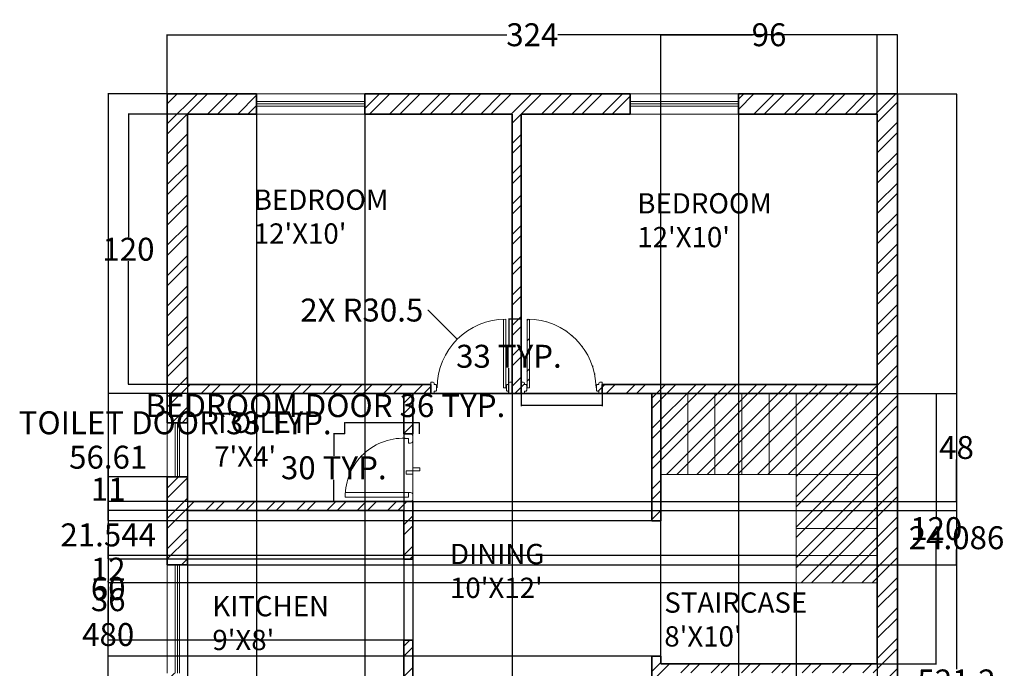
# Model space of a CAD drawing. Units: inches. Extents: x 2025 to 2472, y 2991 to 3578.
# Tile 2 of 2: x 2025 to 2462, y 3291 to 3578. Entities that reach past the tile are written whole.
import ezdxf

# ---------------------------------------------------------------- set-up
doc = ezdxf.new("R2010")
doc.units = ezdxf.units.IN
for name, color, linetype, lineweight in [('00 FURNITURE', 15, 'Continuous', 15), ('A-ANNO-DIMS', 2, 'Continuous', 18), ('A-AREA-IDEN', 7, 'Continuous', 18), ('A-DOOR', 4, 'Continuous', 18), ('A-FLOR-STRS', 7, 'Continuous', 18), ('A-WALL-PATT', 252, 'Continuous', 13), ('A_FUR 1', 5, 'Continuous', 5), ('WALL', 7, 'Continuous', 35), ('WINDOW', 160, 'Continuous', 13)]:
    doc.layers.add(name, color=color, linetype=linetype, lineweight=lineweight)
doc.styles.get("Standard").update_dxf_attribs({"font": 'arial.ttf'})
doc.dimstyles.get("Standard").update_dxf_attribs({"dimtxt": 10.18, "dimasz": 0.18, "dimexe": 0.18, "dimexo": 0.0625, "dimgap": 0.09, "dimtad": 0, "dimtih": 1, "dimtoh": 1, "dimdec": 0, "dimzin": 0, "dimdsep": 46, "dimlunit": 3, "dimtxsty": 'Standard', "dimcen": 0.09, "dimadec": 0, "dimazin": 0, "dimtfac": 1, "dimtdec": 0, "dimtofl": 0, "dimtmove": 0, "dimatfit": 3, "dimfxl": 1, "dimtolj": 1, "dimtzin": 0, "dimarcsym": 0})

# ---------------------------------------------------------------- blocks, each defined once
blk = doc.blocks.new('DDD')
at = {"layer": '00 FURNITURE'}
for p, q in [((-12579.77, -15859.53), (-12579.77, -15829.05)), ((-12578.77, -15859.53), (-12578.77, -15829.03)), ((-12612.02, -15857.03), (-12612.02, -15862.03)), ((-12611.02, -15857.03), (-12612.02, -15857.03)), ((-12610.52, -15858.03), (-12610.52, -15857.53)), ((-12577.52, -15858.03), (-12577.52, -15857.53)), ((-12577.02, -15857.03), (-12576.02, -15857.03)), ((-12576.02, -15857.03), (-12576.02, -15862.03)), ((-12612.02, -15862.03), (-12611.02, -15862.03)), ((-12610.52, -15861.53), (-12610.52, -15861.03)), ((-12578.77, -15859.53), (-12579.77, -15859.53)), ((-12577.52, -15861.53), (-12577.52, -15861.03)), ((-12576.02, -15862.03), (-12577.02, -15862.03))]:
    blk.add_line(p, q, dxfattribs=at)
for points in [[(-12610.52, -15861.03), (-12610.02, -15861.03, 0.414214), (-12609.52, -15860.53), (-12609.52, -15858.53, 0.414214), (-12610.02, -15858.03), (-12610.52, -15858.03)], [(-12577.52, -15861.03), (-12578.02, -15861.03, -0.414214), (-12578.52, -15860.53), (-12578.52, -15858.53, -0.414214), (-12578.02, -15858.03), (-12577.52, -15858.03)]]:
    blk.add_lwpolyline(points, format="xyb", dxfattribs=at)
for centre, radius, start, end in [((-12578.77, -15859.53), 30.5, 90, 180), ((-12611.02, -15857.53), 0.5, 0, 90), ((-12577.02, -15857.53), 0.5, 90, 180), ((-12611.02, -15861.53), 0.5, 270, 0), ((-12577.02, -15861.53), 0.5, 180, 270)]:
    blk.add_arc(centre, radius, start, end, dxfattribs=at)
blk = doc.blocks.new('ESTSET')
at = {"layer": 'A_FUR 1'}
for p, q in [((-10.44, 4.1), (-10.44, 32.1)), ((-8.44, 4.1), (-8.44, 32.1)), ((-36.44, 6.1), (-36.44, 3.1)), ((-34.44, 6.1), (-36.44, 6.1)), ((-34.44, 4.1), (-34.44, 6.1)), ((-34.44, 4.1), (-34.44, 6.1)), ((-8.44, 4.1), (-8.44, 6.1)), ((-8.44, 6.1), (-6.44, 6.1)), ((-8.44, 4.1), (-8.44, 6.1)), ((-6.44, 6.1), (-6.44, 3.1)), ((-6.44, 2.1), (-36.44, 2.1)), ((-35.44, 2.1), (-33.44, 2.1)), ((-32.44, 4.1), (-34.44, 4.1)), ((-32.44, 4.1), (-34.44, 4.1)), ((-32.44, 3.1), (-32.44, 4.1)), ((-10.44, 3.1), (-10.44, 4.1)), ((-10.44, 4.1), (-8.44, 4.1)), ((-10.44, 4.1), (-8.44, 4.1)), ((-7.44, 2.1), (-9.44, 2.1))]:
    blk.add_line(p, q, dxfattribs=at)
for points in [[(-21.44, 2.1), (-18.67, 2.1), (-18.67, 5.1), (-20.06, 5.1)], [(-20.06, 5.1), (-20.06, -0.91)], [(-21.44, 2.1), (-21.44, -0.91), (-20.06, -0.91)]]:
    blk.add_lwpolyline(points, dxfattribs=at)
for centre, radius, start, end in [((-8.91, 6.46), 25.64, 88.9606, 185.2816), ((-35.44, 3.1), 1, 180, 270), ((-33.44, 3.1), 1, 270, 0), ((-9.44, 3.1), 1, 180, 270), ((-7.44, 3.1), 1, 270, 0)]:
    blk.add_arc(centre, radius, start, end, dxfattribs=at)
blk = doc.blocks.new('WIN-48IN')
for p, q in [((48, 9), (0, 9)), ((48, 5.5), (0, 5.5)), ((48, 4.5), (0, 4.5)), ((48, 3.5), (0, 3.5)), ((0, 0), (48, 0))]:
    blk.add_line(p, q)
blk = doc.blocks.new('WIN-24IN')
for p, q in [((3.5, 24), (3.5, 0)), ((4.5, 24), (4.5, 0)), ((5.5, 24), (5.5, 0))]:
    blk.add_line(p, q)
blk.add_lwpolyline([(0, 0), (9, 0), (9, 24), (0, 24)], close=True)
blk = doc.blocks.new('*D10')
at = {"layer": 'A-ANNO-DIMS', "color": 0, "lineweight": -2, "transparency": 16777216}
for p, q in [((2247.79, 3412.44), (2247.79, 3406.92)), ((2283.79, 3412.44), (2283.79, 3406.92)), ((2247.79, 3407.1), (2247.61, 3407.1)), ((2283.61, 3407.1), (2247.97, 3407.1))]:
    blk.add_line(p, q, dxfattribs=at)
at = {"layer": 'A-ANNO-DIMS', "color": 0, "transparency": 16777216}
for points in [[(2247.97, 3407.13), (2247.97, 3407.07), (2247.79, 3407.1)], [(2283.61, 3407.13), (2283.61, 3407.07), (2283.79, 3407.1)]]:
    blk.add_solid(points, dxfattribs=at)
at = {"layer": 'Defpoints', "color": 0, "transparency": 16777216}
for p in [(2247.79, 3412.5), (2283.79, 3412.5), (2247.79, 3407.1)]:
    blk.add_point(p, dxfattribs=at)
at = {"layer": 'A-ANNO-DIMS', "color": 0, "transparency": 16777216, "insert": (2160.94, 3407.1), "char_height": 10.18, "attachment_point": 5}
blk.add_mtext('\\A1;BEDROOM DOOR 36 TYP.', dxfattribs=at)
blk = doc.blocks.new('*D11')
at = {"layer": 'A-ANNO-DIMS', "color": 0, "lineweight": -2, "transparency": 16777216}
for p, q in [((2247.72, 3445.5), (2242.21, 3445.5)), ((2242.39, 3445.32), (2242.39, 3434.29)), ((2242.39, 3412.68), (2242.39, 3423.71)), ((2247.72, 3412.5), (2242.21, 3412.5))]:
    blk.add_line(p, q, dxfattribs=at)
at = {"layer": 'A-ANNO-DIMS', "color": 0, "transparency": 16777216}
for points in [[(2242.36, 3445.32), (2242.42, 3445.32), (2242.39, 3445.5)], [(2242.36, 3412.68), (2242.42, 3412.68), (2242.39, 3412.5)]]:
    blk.add_solid(points, dxfattribs=at)
at = {"layer": 'Defpoints', "color": 0, "transparency": 16777216}
for p in [(2242.39, 3445.5), (2247.79, 3445.5), (2247.79, 3412.5)]:
    blk.add_point(p, dxfattribs=at)
at = {"layer": 'A-ANNO-DIMS', "color": 0, "transparency": 16777216, "insert": (2242.39, 3429), "char_height": 10.18, "attachment_point": 5}
blk.add_mtext('\\A1;33 TYP.', dxfattribs=at)
blk = doc.blocks.new('*D12')
at = {"layer": 'A-ANNO-DIMS', "color": 0, "lineweight": -2, "transparency": 16777216}
for p, q in [((2169.65, 3399.47), (2169.47, 3399.47)), ((2169.65, 3394.56), (2169.65, 3399.65)), ((2202.61, 3399.47), (2169.83, 3399.47)), ((2202.79, 3394.56), (2202.79, 3399.65))]:
    blk.add_line(p, q, dxfattribs=at)
at = {"layer": 'A-ANNO-DIMS', "color": 0, "transparency": 16777216}
for points in [[(2169.83, 3399.5), (2169.83, 3399.44), (2169.65, 3399.47)], [(2202.61, 3399.5), (2202.61, 3399.44), (2202.79, 3399.47)]]:
    blk.add_solid(points, dxfattribs=at)
at = {"layer": 'Defpoints', "color": 0, "transparency": 16777216}
for p in [(2169.65, 3399.47), (2169.65, 3394.5), (2202.79, 3394.5)]:
    blk.add_point(p, dxfattribs=at)
at = {"layer": 'A-ANNO-DIMS', "color": 0, "transparency": 16777216, "insert": (2094.3, 3399.47), "char_height": 10.18, "attachment_point": 5}
blk.add_mtext('\\A1;TOILET DOOR 33 TYP.', dxfattribs=at)
blk = doc.blocks.new('*D13')
at = {"layer": 'A-ANNO-DIMS', "color": 0, "lineweight": -2, "transparency": 16777216}
for p, q in [((2169.59, 3394.5), (2164.5, 3394.5)), ((2164.68, 3394.32), (2164.68, 3384.79)), ((2164.68, 3364.68), (2164.68, 3374.21)), ((2169.59, 3364.5), (2164.5, 3364.5))]:
    blk.add_line(p, q, dxfattribs=at)
at = {"layer": 'A-ANNO-DIMS', "color": 0, "transparency": 16777216}
for points in [[(2164.65, 3394.32), (2164.71, 3394.32), (2164.68, 3394.5)], [(2164.65, 3364.68), (2164.71, 3364.68), (2164.68, 3364.5)]]:
    blk.add_solid(points, dxfattribs=at)
at = {"layer": 'Defpoints', "color": 0, "transparency": 16777216}
for p in [(2169.65, 3394.5), (2164.68, 3364.5), (2169.65, 3364.5)]:
    blk.add_point(p, dxfattribs=at)
at = {"layer": 'A-ANNO-DIMS', "color": 0, "transparency": 16777216, "insert": (2164.68, 3379.5), "char_height": 10.18, "attachment_point": 5}
blk.add_mtext('\\A1;30 TYP.', dxfattribs=at)
blk = doc.blocks.new('*D14')
at = {"layer": 'A-ANNO-DIMS', "color": 0, "lineweight": -2, "transparency": 16777216}
for p, q in [((2090.79, 3545.56), (2090.79, 3571.88)), ((2090.97, 3571.7), (2241.47, 3571.7)), ((2414.61, 3571.7), (2264.1, 3571.7)), ((2414.79, 3545.56), (2414.79, 3571.88))]:
    blk.add_line(p, q, dxfattribs=at)
at = {"layer": 'A-ANNO-DIMS', "color": 0, "transparency": 16777216}
for points in [[(2090.97, 3571.73), (2090.97, 3571.67), (2090.79, 3571.7)], [(2414.61, 3571.73), (2414.61, 3571.67), (2414.79, 3571.7)]]:
    blk.add_solid(points, dxfattribs=at)
at = {"layer": 'Defpoints', "color": 0, "transparency": 16777216}
for p in [(2414.79, 3571.7), (2090.79, 3545.5), (2414.79, 3545.5)]:
    blk.add_point(p, dxfattribs=at)
at = {"layer": 'A-ANNO-DIMS', "color": 0, "transparency": 16777216, "insert": (2252.79, 3571.7), "char_height": 10.18, "attachment_point": 5}
blk.add_mtext('\\A1;324', dxfattribs=at)
blk = doc.blocks.new('*D15')
at = {"layer": 'A-ANNO-DIMS', "color": 0, "lineweight": -2, "transparency": 16777216}
for p, q in [((2414.85, 3545.5), (2441.17, 3545.5)), ((2440.99, 3545.32), (2440.99, 3290.19)), ((2440.99, 3024.48), (2440.99, 3279.61)), ((2267.85, 3024.3), (2441.17, 3024.3))]:
    blk.add_line(p, q, dxfattribs=at)
at = {"layer": 'A-ANNO-DIMS', "color": 0, "transparency": 16777216}
for points in [[(2440.96, 3545.32), (2441.02, 3545.32), (2440.99, 3545.5)], [(2440.96, 3024.48), (2441.02, 3024.48), (2440.99, 3024.3)]]:
    blk.add_solid(points, dxfattribs=at)
at = {"layer": 'Defpoints', "color": 0, "transparency": 16777216}
for p in [(2414.79, 3545.5), (2440.99, 3545.5), (2267.79, 3024.3)]:
    blk.add_point(p, dxfattribs=at)
at = {"layer": 'A-ANNO-DIMS', "color": 0, "transparency": 16777216, "insert": (2440.99, 3284.9), "char_height": 10.18, "attachment_point": 5}
blk.add_mtext('\\A1;521.2', dxfattribs=at)
blk = doc.blocks.new('*D16')
at = {"layer": 'A-ANNO-DIMS', "color": 0, "lineweight": -2, "transparency": 16777216}
for p, q in [((2090.72, 3545.5), (2064.41, 3545.5)), ((2064.59, 3545.32), (2064.59, 3310.79)), ((2064.59, 3065.68), (2064.59, 3300.21)), ((2090.72, 3065.5), (2064.41, 3065.5))]:
    blk.add_line(p, q, dxfattribs=at)
at = {"layer": 'A-ANNO-DIMS', "color": 0, "transparency": 16777216}
for points in [[(2064.56, 3545.32), (2064.62, 3545.32), (2064.59, 3545.5)], [(2064.56, 3065.68), (2064.62, 3065.68), (2064.59, 3065.5)]]:
    blk.add_solid(points, dxfattribs=at)
at = {"layer": 'Defpoints', "color": 0, "transparency": 16777216}
for p in [(2064.59, 3545.5), (2090.79, 3545.5), (2090.79, 3065.5)]:
    blk.add_point(p, dxfattribs=at)
at = {"layer": 'A-ANNO-DIMS', "color": 0, "transparency": 16777216, "insert": (2064.59, 3305.5), "char_height": 10.18, "attachment_point": 5}
blk.add_mtext('\\A1;480', dxfattribs=at)
blk = doc.blocks.new('*D18')
at = {"layer": 'A-ANNO-DIMS', "color": 0, "lineweight": -2, "transparency": 16777216}
for p, q in [((2099.79, 3536.44), (2099.79, 2997.92)), ((2130.46, 3536.44), (2130.46, 2997.92)), ((2099.97, 2998.1), (2130.28, 2998.1)), ((2130.46, 2998.1), (2130.64, 2998.1))]:
    blk.add_line(p, q, dxfattribs=at)
at = {"layer": 'A-ANNO-DIMS', "color": 0, "transparency": 16777216}
for points in [[(2099.97, 2998.13), (2099.97, 2998.07), (2099.79, 2998.1)], [(2130.28, 2998.13), (2130.28, 2998.07), (2130.46, 2998.1)]]:
    blk.add_solid(points, dxfattribs=at)
at = {"layer": 'Defpoints', "color": 0, "transparency": 16777216}
for p in [(2099.79, 3536.5), (2130.46, 3536.5), (2130.46, 2998.1)]:
    blk.add_point(p, dxfattribs=at)
at = {"layer": 'A-ANNO-DIMS', "color": 0, "transparency": 16777216, "insert": (2151.86, 2998.1), "char_height": 10.18, "attachment_point": 5}
blk.add_mtext('\\A1;30.676', dxfattribs=at)
blk = doc.blocks.new('*D19')
at = {"layer": 'A-ANNO-DIMS', "color": 0, "lineweight": -2, "transparency": 16777216}
for p, q in [((2178.46, 3536.44), (2178.46, 2997.92)), ((2243.79, 3536.44), (2243.79, 2997.92)), ((2178.64, 2998.1), (2193.88, 2998.1)), ((2243.61, 2998.1), (2228.37, 2998.1))]:
    blk.add_line(p, q, dxfattribs=at)
at = {"layer": 'A-ANNO-DIMS', "color": 0, "transparency": 16777216}
for points in [[(2178.64, 2998.13), (2178.64, 2998.07), (2178.46, 2998.1)], [(2243.61, 2998.13), (2243.61, 2998.07), (2243.79, 2998.1)]]:
    blk.add_solid(points, dxfattribs=at)
at = {"layer": 'Defpoints', "color": 0, "transparency": 16777216}
for p in [(2178.46, 3536.5), (2243.79, 3536.5), (2243.79, 2998.1)]:
    blk.add_point(p, dxfattribs=at)
at = {"layer": 'A-ANNO-DIMS', "color": 0, "transparency": 16777216, "insert": (2211.12, 2998.1), "char_height": 10.18, "attachment_point": 5}
blk.add_mtext('\\A1;65.32', dxfattribs=at)
blk = doc.blocks.new('*D20')
at = {"layer": 'A-ANNO-DIMS', "color": 0, "lineweight": -2, "transparency": 16777216}
for p, q in [((2344.19, 3536.44), (2344.19, 2997.92)), ((2405.79, 3536.44), (2405.79, 2997.92)), ((2344.37, 2998.1), (2361.65, 2998.1)), ((2405.61, 2998.1), (2388.32, 2998.1))]:
    blk.add_line(p, q, dxfattribs=at)
at = {"layer": 'A-ANNO-DIMS', "color": 0, "transparency": 16777216}
for points in [[(2344.37, 2998.13), (2344.37, 2998.07), (2344.19, 2998.1)], [(2405.61, 2998.13), (2405.61, 2998.07), (2405.79, 2998.1)]]:
    blk.add_solid(points, dxfattribs=at)
at = {"layer": 'Defpoints', "color": 0, "transparency": 16777216}
for p in [(2344.19, 3536.5), (2405.79, 3536.5), (2405.79, 2998.1)]:
    blk.add_point(p, dxfattribs=at)
at = {"layer": 'A-ANNO-DIMS', "color": 0, "transparency": 16777216, "insert": (2374.99, 2998.1), "char_height": 10.18, "attachment_point": 5}
blk.add_mtext('\\A1;61.6', dxfattribs=at)
blk = doc.blocks.new('*D26')
at = {"layer": 'A-ANNO-DIMS', "color": 0, "lineweight": -2, "transparency": 16777216}
for p, q in [((2099.72, 3536.5), (2073.41, 3536.5)), ((2073.59, 3536.32), (2073.59, 3481.79)), ((2073.59, 3416.68), (2073.59, 3471.21)), ((2099.72, 3416.5), (2073.41, 3416.5))]:
    blk.add_line(p, q, dxfattribs=at)
at = {"layer": 'A-ANNO-DIMS', "color": 0, "transparency": 16777216}
for points in [[(2073.56, 3536.32), (2073.62, 3536.32), (2073.59, 3536.5)], [(2073.56, 3416.68), (2073.62, 3416.68), (2073.59, 3416.5)]]:
    blk.add_solid(points, dxfattribs=at)
at = {"layer": 'Defpoints', "color": 0, "transparency": 16777216}
for p in [(2073.59, 3536.5), (2099.79, 3536.5), (2099.79, 3416.5)]:
    blk.add_point(p, dxfattribs=at)
at = {"layer": 'A-ANNO-DIMS', "color": 0, "transparency": 16777216, "insert": (2073.59, 3476.5), "char_height": 10.18, "attachment_point": 5}
blk.add_mtext('\\A1;120', dxfattribs=at)
blk = doc.blocks.new('*D28')
at = {"layer": 'A-ANNO-DIMS', "color": 0, "lineweight": -2, "transparency": 16777216}
for p, q in [((2099.85, 3360.5), (2441.17, 3360.5)), ((2440.99, 3360.32), (2440.99, 3353.75)), ((2440.99, 3336.6), (2440.99, 3343.17)), ((2099.85, 3336.42), (2441.17, 3336.42))]:
    blk.add_line(p, q, dxfattribs=at)
at = {"layer": 'A-ANNO-DIMS', "color": 0, "transparency": 16777216}
for points in [[(2440.96, 3360.32), (2441.02, 3360.32), (2440.99, 3360.5)], [(2440.96, 3336.6), (2441.02, 3336.6), (2440.99, 3336.42)]]:
    blk.add_solid(points, dxfattribs=at)
at = {"layer": 'Defpoints', "color": 0, "transparency": 16777216}
for p in [(2099.79, 3360.5), (2440.99, 3360.5), (2099.79, 3336.42)]:
    blk.add_point(p, dxfattribs=at)
at = {"layer": 'A-ANNO-DIMS', "color": 0, "transparency": 16777216, "insert": (2440.99, 3348.46), "char_height": 10.18, "attachment_point": 5}
blk.add_mtext('\\A1;24.086', dxfattribs=at)
blk = doc.blocks.new('*D29')
at = {"layer": 'A-ANNO-DIMS', "color": 0, "lineweight": -2, "transparency": 16777216}
for p, q in [((2090.72, 3375.5), (2064.41, 3375.5)), ((2064.59, 3375.32), (2064.59, 3375.2)), ((2099.72, 3364.5), (2064.41, 3364.5)), ((2064.59, 3364.68), (2064.59, 3364.8))]:
    blk.add_line(p, q, dxfattribs=at)
at = {"layer": 'A-ANNO-DIMS', "color": 0, "transparency": 16777216}
for points in [[(2064.56, 3375.32), (2064.62, 3375.32), (2064.59, 3375.5)], [(2064.56, 3364.68), (2064.62, 3364.68), (2064.59, 3364.5)]]:
    blk.add_solid(points, dxfattribs=at)
at = {"layer": 'Defpoints', "color": 0, "transparency": 16777216}
for p in [(2090.79, 3375.5), (2064.59, 3364.5), (2099.79, 3364.5)]:
    blk.add_point(p, dxfattribs=at)
at = {"layer": 'A-ANNO-DIMS', "color": 0, "transparency": 16777216, "insert": (2064.59, 3370), "char_height": 10.18, "attachment_point": 5}
blk.add_mtext('\\A1;11', dxfattribs=at)
blk = doc.blocks.new('*D31')
at = {"layer": 'A-ANNO-DIMS', "color": 0, "lineweight": -2, "transparency": 16777216}
for p, q in [((2099.79, 3412.44), (2099.79, 2997.92)), ((2195.79, 3412.44), (2195.79, 2997.92)), ((2099.97, 2998.1), (2140.41, 2998.1)), ((2195.61, 2998.1), (2155.16, 2998.1))]:
    blk.add_line(p, q, dxfattribs=at)
at = {"layer": 'A-ANNO-DIMS', "color": 0, "transparency": 16777216}
for points in [[(2099.97, 2998.13), (2099.97, 2998.07), (2099.79, 2998.1)], [(2195.61, 2998.13), (2195.61, 2998.07), (2195.79, 2998.1)]]:
    blk.add_solid(points, dxfattribs=at)
at = {"layer": 'Defpoints', "color": 0, "transparency": 16777216}
for p in [(2099.79, 3412.5), (2195.79, 3412.5), (2195.79, 2998.1)]:
    blk.add_point(p, dxfattribs=at)
at = {"layer": 'A-ANNO-DIMS', "color": 0, "transparency": 16777216, "insert": (2147.79, 2998.1), "char_height": 10.18, "attachment_point": 5}
blk.add_mtext('\\A1;96', dxfattribs=at)
blk = doc.blocks.new('*D32')
at = {"layer": 'A-ANNO-DIMS', "color": 0, "lineweight": -2, "transparency": 16777216}
for p, q in [((2099.85, 3412.5), (2441.17, 3412.5)), ((2440.99, 3412.32), (2440.99, 3393.79)), ((2440.99, 3364.68), (2440.99, 3383.21)), ((2099.85, 3364.5), (2441.17, 3364.5))]:
    blk.add_line(p, q, dxfattribs=at)
at = {"layer": 'A-ANNO-DIMS', "color": 0, "transparency": 16777216}
for points in [[(2440.96, 3412.32), (2441.02, 3412.32), (2440.99, 3412.5)], [(2440.96, 3364.68), (2441.02, 3364.68), (2440.99, 3364.5)]]:
    blk.add_solid(points, dxfattribs=at)
at = {"layer": 'Defpoints', "color": 0, "transparency": 16777216}
for p in [(2099.79, 3412.5), (2440.99, 3412.5), (2099.79, 3364.5)]:
    blk.add_point(p, dxfattribs=at)
at = {"layer": 'A-ANNO-DIMS', "color": 0, "transparency": 16777216, "insert": (2440.99, 3388.5), "char_height": 10.18, "attachment_point": 5}
blk.add_mtext('\\A1;48', dxfattribs=at)
blk = doc.blocks.new('*D33')
at = {"layer": 'A-ANNO-DIMS', "color": 0, "lineweight": -2, "transparency": 16777216}
for p, q in [((2309.79, 3292.56), (2309.79, 3571.88)), ((2309.97, 3571.7), (2350.41, 3571.7)), ((2405.61, 3571.7), (2365.16, 3571.7)), ((2405.79, 3292.56), (2405.79, 3571.88))]:
    blk.add_line(p, q, dxfattribs=at)
at = {"layer": 'A-ANNO-DIMS', "color": 0, "transparency": 16777216}
for points in [[(2309.97, 3571.73), (2309.97, 3571.67), (2309.79, 3571.7)], [(2405.61, 3571.73), (2405.61, 3571.67), (2405.79, 3571.7)]]:
    blk.add_solid(points, dxfattribs=at)
at = {"layer": 'Defpoints', "color": 0, "transparency": 16777216}
for p in [(2405.79, 3571.7), (2309.79, 3292.5), (2405.79, 3292.5)]:
    blk.add_point(p, dxfattribs=at)
at = {"layer": 'A-ANNO-DIMS', "color": 0, "transparency": 16777216, "insert": (2357.79, 3571.7), "char_height": 10.18, "attachment_point": 5}
blk.add_mtext('\\A1;96', dxfattribs=at)
blk = doc.blocks.new('*D34')
at = {"layer": 'A-ANNO-DIMS', "color": 0, "lineweight": -2, "transparency": 16777216}
for p, q in [((2405.85, 3412.5), (2432.17, 3412.5)), ((2431.99, 3412.32), (2431.99, 3357.79)), ((2431.99, 3292.68), (2431.99, 3347.21)), ((2405.85, 3292.5), (2432.17, 3292.5))]:
    blk.add_line(p, q, dxfattribs=at)
at = {"layer": 'A-ANNO-DIMS', "color": 0, "transparency": 16777216}
for points in [[(2431.96, 3412.32), (2432.02, 3412.32), (2431.99, 3412.5)], [(2431.96, 3292.68), (2432.02, 3292.68), (2431.99, 3292.5)]]:
    blk.add_solid(points, dxfattribs=at)
at = {"layer": 'Defpoints', "color": 0, "transparency": 16777216}
for p in [(2405.79, 3412.5), (2405.79, 3292.5), (2431.99, 3292.5)]:
    blk.add_point(p, dxfattribs=at)
at = {"layer": 'A-ANNO-DIMS', "color": 0, "transparency": 16777216, "insert": (2431.99, 3352.5), "char_height": 10.18, "attachment_point": 5}
blk.add_mtext('\\A1;120', dxfattribs=at)
blk = doc.blocks.new('*D36')
at = {"layer": 'A-ANNO-DIMS', "color": 0, "lineweight": -2, "transparency": 16777216}
for p, q in [((2195.72, 3338.96), (2064.41, 3338.96)), ((2064.59, 3338.78), (2064.59, 3326.25)), ((2064.59, 3303.14), (2064.59, 3315.67)), ((2195.72, 3302.96), (2064.41, 3302.96))]:
    blk.add_line(p, q, dxfattribs=at)
at = {"layer": 'A-ANNO-DIMS', "color": 0, "transparency": 16777216}
for points in [[(2064.56, 3338.78), (2064.62, 3338.78), (2064.59, 3338.96)], [(2064.56, 3303.14), (2064.62, 3303.14), (2064.59, 3302.96)]]:
    blk.add_solid(points, dxfattribs=at)
at = {"layer": 'Defpoints', "color": 0, "transparency": 16777216}
for p in [(2195.79, 3338.96), (2064.59, 3302.96), (2195.79, 3302.96)]:
    blk.add_point(p, dxfattribs=at)
at = {"layer": 'A-ANNO-DIMS', "color": 0, "transparency": 16777216, "insert": (2064.59, 3320.96), "char_height": 10.18, "attachment_point": 5}
blk.add_mtext('\\A1;36', dxfattribs=at)
blk = doc.blocks.new('*D37')
at = {"layer": 'A-ANNO-DIMS', "color": 0, "lineweight": -2, "transparency": 16777216}
for p, q in [((2195.72, 3360.5), (2064.41, 3360.5)), ((2064.59, 3360.32), (2064.59, 3355.02)), ((2064.59, 3339.14), (2064.59, 3344.44)), ((2195.72, 3338.96), (2064.41, 3338.96))]:
    blk.add_line(p, q, dxfattribs=at)
at = {"layer": 'A-ANNO-DIMS', "color": 0, "transparency": 16777216}
for points in [[(2064.56, 3360.32), (2064.62, 3360.32), (2064.59, 3360.5)], [(2064.56, 3339.14), (2064.62, 3339.14), (2064.59, 3338.96)]]:
    blk.add_solid(points, dxfattribs=at)
at = {"layer": 'Defpoints', "color": 0, "transparency": 16777216}
for p in [(2195.79, 3360.5), (2064.59, 3338.96), (2195.79, 3338.96)]:
    blk.add_point(p, dxfattribs=at)
at = {"layer": 'A-ANNO-DIMS', "color": 0, "transparency": 16777216, "insert": (2064.59, 3349.73), "char_height": 10.18, "attachment_point": 5}
blk.add_mtext('\\A1;21.544', dxfattribs=at)
blk = doc.blocks.new('*D39')
at = {"layer": 'A-ANNO-DIMS', "color": 0, "lineweight": -2, "transparency": 16777216}
for p, q in [((2305.72, 3355.89), (2064.41, 3355.89)), ((2064.59, 3355.71), (2064.59, 3331.18)), ((2064.59, 3296.07), (2064.59, 3320.61)), ((2305.72, 3295.89), (2064.41, 3295.89))]:
    blk.add_line(p, q, dxfattribs=at)
at = {"layer": 'A-ANNO-DIMS', "color": 0, "transparency": 16777216}
for points in [[(2064.56, 3355.71), (2064.62, 3355.71), (2064.59, 3355.89)], [(2064.56, 3296.07), (2064.62, 3296.07), (2064.59, 3295.89)]]:
    blk.add_solid(points, dxfattribs=at)
at = {"layer": 'Defpoints', "color": 0, "transparency": 16777216}
for p in [(2064.59, 3355.89), (2305.79, 3355.89), (2305.79, 3295.89)]:
    blk.add_point(p, dxfattribs=at)
at = {"layer": 'A-ANNO-DIMS', "color": 0, "transparency": 16777216, "insert": (2064.59, 3325.89), "char_height": 10.18, "attachment_point": 5}
blk.add_mtext('\\A1;60', dxfattribs=at)
blk = doc.blocks.new('*D40')
at = {"layer": 'A-ANNO-DIMS', "color": 0, "lineweight": -2, "transparency": 16777216}
for p, q in [((2309.72, 3412.5), (2064.41, 3412.5)), ((2064.59, 3412.32), (2064.59, 3389.49)), ((2064.59, 3356.07), (2064.59, 3378.91)), ((2305.72, 3355.89), (2064.41, 3355.89))]:
    blk.add_line(p, q, dxfattribs=at)
at = {"layer": 'A-ANNO-DIMS', "color": 0, "transparency": 16777216}
for points in [[(2064.56, 3412.32), (2064.62, 3412.32), (2064.59, 3412.5)], [(2064.56, 3356.07), (2064.62, 3356.07), (2064.59, 3355.89)]]:
    blk.add_solid(points, dxfattribs=at)
at = {"layer": 'Defpoints', "color": 0, "transparency": 16777216}
for p in [(2064.59, 3412.5), (2309.79, 3412.5), (2305.79, 3355.89)]:
    blk.add_point(p, dxfattribs=at)
at = {"layer": 'A-ANNO-DIMS', "color": 0, "transparency": 16777216, "insert": (2064.59, 3384.2), "char_height": 10.18, "attachment_point": 5}
blk.add_mtext('\\A1;56.61', dxfattribs=at)
blk = doc.blocks.new('*D41')
at = {"layer": 'A-ANNO-DIMS', "color": 0, "lineweight": -2, "transparency": 16777216}
for p, q in [((2195.79, 3360.44), (2195.79, 2997.92)), ((2199.79, 3338.9), (2199.79, 2997.92)), ((2195.97, 2998.1), (2199.61, 2998.1)), ((2199.79, 2998.1), (2199.97, 2998.1))]:
    blk.add_line(p, q, dxfattribs=at)
at = {"layer": 'A-ANNO-DIMS', "color": 0, "transparency": 16777216}
for points in [[(2195.97, 2998.13), (2195.97, 2998.07), (2195.79, 2998.1)], [(2199.61, 2998.13), (2199.61, 2998.07), (2199.79, 2998.1)]]:
    blk.add_solid(points, dxfattribs=at)
at = {"layer": 'Defpoints', "color": 0, "transparency": 16777216}
for p in [(2195.79, 3360.5), (2199.79, 3338.96), (2199.79, 2998.1)]:
    blk.add_point(p, dxfattribs=at)
at = {"layer": 'A-ANNO-DIMS', "color": 0, "transparency": 16777216, "insert": (2203.58, 2998.1), "char_height": 10.18, "attachment_point": 5}
blk.add_mtext('\\A1;4', dxfattribs=at)
blk = doc.blocks.new('*D42')
at = {"layer": 'A-ANNO-DIMS', "color": 0, "lineweight": -2, "transparency": 16777216}
for p, q in [((2369.79, 3328.44), (2369.79, 2997.92)), ((2405.79, 3328.44), (2405.79, 2997.92)), ((2369.97, 2998.1), (2380.41, 2998.1)), ((2405.61, 2998.1), (2395.16, 2998.1))]:
    blk.add_line(p, q, dxfattribs=at)
at = {"layer": 'A-ANNO-DIMS', "color": 0, "transparency": 16777216}
for points in [[(2369.97, 2998.13), (2369.97, 2998.07), (2369.79, 2998.1)], [(2405.61, 2998.13), (2405.61, 2998.07), (2405.79, 2998.1)]]:
    blk.add_solid(points, dxfattribs=at)
at = {"layer": 'Defpoints', "color": 0, "transparency": 16777216}
for p in [(2369.79, 3328.5), (2405.79, 3328.5), (2405.79, 2998.1)]:
    blk.add_point(p, dxfattribs=at)
at = {"layer": 'A-ANNO-DIMS', "color": 0, "transparency": 16777216, "insert": (2387.79, 2998.1), "char_height": 10.18, "attachment_point": 5}
blk.add_mtext('\\A1;36', dxfattribs=at)
blk = doc.blocks.new('*D43')
at = {"layer": 'A-ANNO-DIMS', "color": 0, "lineweight": -2, "transparency": 16777216}
for p, q in [((2369.72, 3340.5), (2064.41, 3340.5)), ((2064.59, 3340.32), (2064.59, 3339.7)), ((2064.59, 3328.68), (2064.59, 3329.3)), ((2369.72, 3328.5), (2064.41, 3328.5))]:
    blk.add_line(p, q, dxfattribs=at)
at = {"layer": 'A-ANNO-DIMS', "color": 0, "transparency": 16777216}
for points in [[(2064.56, 3340.32), (2064.62, 3340.32), (2064.59, 3340.5)], [(2064.56, 3328.68), (2064.62, 3328.68), (2064.59, 3328.5)]]:
    blk.add_solid(points, dxfattribs=at)
at = {"layer": 'Defpoints', "color": 0, "transparency": 16777216}
for p in [(2064.59, 3340.5), (2369.79, 3340.5), (2369.79, 3328.5)]:
    blk.add_point(p, dxfattribs=at)
at = {"layer": 'A-ANNO-DIMS', "color": 0, "transparency": 16777216, "insert": (2064.59, 3334.5), "char_height": 10.18, "attachment_point": 5}
blk.add_mtext('\\A1;12', dxfattribs=at)
blk = doc.blocks.new('*D45')
at = {"layer": 'A-ANNO-DIMS', "color": 0, "lineweight": -2, "transparency": 16777216}
for p, q in [((2206.35, 3449.51), (2206.53, 3449.51)), ((2206.53, 3449.51), (2219.34, 3436.7)), ((2240.95, 3415), (2241.13, 3415)), ((2241.04, 3414.91), (2241.04, 3415.09))]:
    blk.add_line(p, q, dxfattribs=at)
at = {"layer": 'A-ANNO-DIMS', "color": 0, "transparency": 16777216}
blk.add_solid([(2219.36, 3436.72), (2219.32, 3436.67), (2219.47, 3436.57)], dxfattribs=at)
at = {"layer": 'Defpoints', "color": 0, "transparency": 16777216}
for p in [(2219.47, 3436.57), (2241.04, 3415)]:
    blk.add_point(p, dxfattribs=at)
at = {"layer": 'A-ANNO-DIMS', "color": 0, "transparency": 16777216, "insert": (2177.1, 3449.51), "char_height": 10.18, "attachment_point": 5}
blk.add_mtext('\\A1;2X R30.5', dxfattribs=at)

msp = doc.modelspace()

# ---------------------------------------------------------------- hatches: boundary and pattern name
at = {"layer": 'A-WALL-PATT'}
h = msp.add_hatch(dxfattribs=at)
h.set_pattern_fill('ANSI32', color=256)
h.paths.add_polyline_path([(2130.4623, 3545.5019), (2090.7862, 3545.5019), (2090.7862, 3399.5018), (2099.7862, 3399.5018), (2099.7862, 3412.5019), (2195.7862, 3412.5019), (2195.7862, 3394.5019), (2199.7862, 3394.5019), (2199.7862, 3412.5019), (2207.7862, 3412.5019), (2207.7862, 3416.5019), (2099.7862, 3416.5019), (2099.7862, 3536.5019), (2130.4623, 3536.5019)])
h.paths.add_polyline_path([(2296.1871, 3545.5019), (2296.187, 3545.5019), (2178.4623, 3545.5019), (2178.4623, 3536.5019), (2243.7862, 3536.5019), (2243.7862, 3417.5019), (2243.7862, 3417.5019), (2243.7862, 3412.5019), (2247.7862, 3412.5019), (2247.7862, 3536.5019), (2296.1871, 3536.5019)])
h.paths.add_polyline_path([(2305.7862, 3236.5019), (2305.7862, 3247.2334), (2305.5512, 3247.2334), (2305.5512, 3252.2334), (2305.7862, 3295.8929), (2309.7862, 3295.8929), (2309.7862, 3292.5019), (2405.7862, 3292.5019), (2405.7862, 3328.5019), (2369.7862, 3328.5019), (2369.7862, 3376.5019), (2309.7862, 3376.5019), (2309.7862, 3355.8929), (2305.7862, 3355.8929), (2305.7862, 3412.5019), (2283.7862, 3412.5019), (2282.7862, 3412.502, -0.41421356), (2282.2862, 3413.002), (2282.2862, 3413.502), (2281.7862, 3413.502, -0.41421356), (2281.2862, 3414.002), (2281.0362, 3415.002, 0.40464108), (2251.5362, 3445.4856), (2251.5362, 3415.002), (2250.2862, 3415.002), (2250.2862, 3414.002, -0.41421356), (2249.7862, 3413.502), (2249.2862, 3413.502), (2249.2862, 3413.002, -0.41421356), (2248.7862, 3412.502), (2247.7862, 3412.502), (2247.7862, 3417.502), (2248.7862, 3417.502, -0.41421356), (2249.2862, 3417.002), (2249.2862, 3416.502), (2249.7862, 3416.502, -0.41421356), (2250.2862, 3416.002), (2250.5362, 3445.502, -0.40734559), (2281.2864, 3415.986, -0.42361429), (2281.7862, 3416.502), (2282.2862, 3416.502), (2282.2862, 3417.002, -0.41421356), (2282.7862, 3417.502), (2283.7862, 3417.502), (2283.7862, 3416.5019), (2405.7862, 3416.5019), (2405.7862, 3536.5019), (2344.1871, 3536.5019), (2344.1871, 3545.5019), (2414.7862, 3545.5019), (2414.7862, 3276.5742), (2414.7861, 3252.5742), (2405.7861, 3252.5742), (2405.7861, 3276.5742), (2405.7862, 3288.5019), (2309.7862, 3288.5019), (2309.7862, 3240.5019), (2375.7543, 3240.5019), (2375.7543, 3240.5021), (2377.648, 3240.5021, -0.42367667), (2403.7543, 3266.5021), (2403.7543, 3240.5021), (2405.7543, 3240.5021), (2405.7543, 3237.5021, -0.41421356), (2404.7543, 3236.5021), (2402.7543, 3236.5021), (2392.14, 3236.5021), (2392.14, 3233.4968), (2390.7543, 3233.4968), (2390.7543, 3236.5021), (2375.7862, 3236.5021), (2375.7862, 3236.5019)])
h.paths.add_polyline_path([(2414.7862, 3252.5742), (2405.7862, 3252.5742), (2405.7862, 3236.5019), (2405.7862, 3074.5019), (2359.7872, 3074.5019), (2359.7872, 3065.5019), (2414.7862, 3065.5019)])
h.paths.add_polyline_path([(2311.7872, 3074.5019), (2311.7872, 3074.5019), (2271.7862, 3074.5019), (2271.7862, 3248.2334), (2271.0512, 3248.2334), (2271.0512, 3247.7334, -0.41421356), (2270.5512, 3247.2334), (2269.5512, 3247.2334), (2269.5512, 3252.5019), (2267.7862, 3252.5019), (2267.7862, 3065.5019), (2311.7872, 3065.5019)])
h.paths.add_polyline_path([(2219.7862, 3074.5019), (2169.7756, 3074.5019), (2169.7756, 3065.502), (2169.7756, 3065.502), (2219.7862, 3065.5019)])
h.paths.add_polyline_path([(2121.7756, 3074.5019), (2099.7862, 3074.5019), (2099.7862, 3152.4991), (2090.7862, 3152.4991), (2090.7862, 3065.5019), (2121.7756, 3065.5019)])
h.paths.add_polyline_path([(2099.7862, 3248.5019), (2231.7862, 3248.5019), (2231.7862, 3252.5019), (2199.7862, 3252.5019), (2199.7862, 3302.9583), (2195.7862, 3302.9583), (2195.7862, 3252.5019), (2099.7862, 3252.5019), (2099.7862, 3288.4156), (2090.7862, 3288.4156), (2090.7862, 3200.4991), (2099.7862, 3200.4991), (2099.7862, 3200.4991)])
h.paths.add_polyline_path([(2099.7862, 3375.5018), (2090.7862, 3375.5018), (2090.7862, 3336.4156), (2099.7862, 3336.4156), (2099.7862, 3336.4156), (2099.7862, 3360.5019), (2195.7862, 3360.5019), (2195.7862, 3338.9583), (2199.7862, 3338.9583), (2199.7862, 3364.5019), (2099.7862, 3364.5019)])

# ---------------------------------------------------------------- linework, layer by layer
at = {"layer": 'A-FLOR-STRS'}
for p, q in [((2321.7862, 3412.5019), (2321.7862, 3376.5019)), ((2333.7862, 3412.5019), (2333.7862, 3376.5019)), ((2345.7862, 3412.5019), (2345.7862, 3376.5019)), ((2357.7862, 3412.5019), (2357.7862, 3376.5019)), ((2369.7862, 3412.5019), (2369.7862, 3328.5019)), ((2309.7862, 3376.5019), (2405.7862, 3376.5019)), ((2369.7862, 3364.5019), (2405.7862, 3364.5019)), ((2369.7862, 3352.5019), (2405.7862, 3352.5019)), ((2369.7862, 3340.5019), (2405.7862, 3340.5019)), ((2369.7862, 3328.5019), (2405.7862, 3328.5019))]:
    msp.add_line(p, q, dxfattribs=at)
at = {"layer": 'WALL'}
for p, q in [((2090.7862, 3545.5019), (2130.4623, 3545.5019)), ((2090.7862, 3399.5018), (2090.7862, 3545.5019)), ((2130.4623, 3545.5019), (2130.4623, 3536.5019)), ((2178.4623, 3545.5019), (2178.4623, 3536.5019)), ((2178.4623, 3545.5019), (2296.1871, 3545.5019)), ((2296.1871, 3545.5019), (2296.1871, 3536.5019)), ((2344.1871, 3545.5019), (2344.1871, 3536.5019)), ((2344.1871, 3545.5019), (2414.7862, 3545.5019)), ((2414.7862, 3545.5019), (2414.7862, 3276.5742)), ((2099.7862, 3536.5019), (2130.4623, 3536.5019)), ((2099.7862, 3416.5019), (2099.7862, 3536.5019)), ((2178.4623, 3536.5019), (2243.7862, 3536.5019)), ((2243.7862, 3412.5019), (2243.7862, 3536.5019)), ((2247.7862, 3412.5019), (2247.7862, 3536.5019)), ((2247.7862, 3536.5019), (2296.1871, 3536.5019)), ((2344.1871, 3536.5019), (2405.7862, 3536.5019)), ((2405.7862, 3536.5019), (2405.7862, 3416.5019)), ((2099.7862, 3416.5019), (2207.7862, 3416.5019)), ((2207.7862, 3412.5019), (2207.7862, 3416.5019)), ((2283.7862, 3416.5019), (2405.7862, 3416.5019)), ((2283.7862, 3412.5019), (2283.7862, 3416.5019)), ((2099.7862, 3412.5019), (2195.7862, 3412.5019)), ((2099.7862, 3399.5018), (2099.7862, 3412.5019)), ((2187.7862, 3412.5019), (2195.7862, 3412.5019)), ((2195.7862, 3394.5019), (2195.7862, 3412.5019)), ((2199.7862, 3412.5019), (2207.7862, 3412.5019)), ((2199.7862, 3412.5019), (2207.7862, 3412.5019)), ((2199.7862, 3412.5019), (2207.7862, 3412.5019)), ((2199.7862, 3394.5019), (2199.7862, 3412.5019)), ((2243.7862, 3412.5019), (2247.7862, 3412.5019)), ((2283.7862, 3412.5019), (2305.7862, 3412.5019)), ((2305.7862, 3412.5019), (2305.7862, 3355.8929)), ((2309.7862, 3412.5019), (2309.7862, 3355.8929)), ((2309.7862, 3412.5019), (2405.7862, 3412.5019)), ((2405.7862, 3412.5019), (2405.7862, 3292.5019)), ((2099.7862, 3399.5018), (2090.7862, 3399.5018)), ((2195.7862, 3394.5019), (2199.7862, 3394.5019)), ((2099.7862, 3375.5018), (2090.7862, 3375.5018)), ((2090.7862, 3336.4156), (2090.7862, 3375.5018)), ((2099.7862, 3364.5019), (2099.7862, 3375.5018)), ((2099.7862, 3364.5019), (2199.7862, 3364.5019)), ((2199.7862, 3338.9583), (2199.7862, 3364.5019)), ((2099.7862, 3360.5019), (2195.7862, 3360.5019)), ((2099.7862, 3336.4156), (2099.7862, 3360.5019)), ((2195.7862, 3338.9583), (2195.7862, 3360.5019)), ((2309.7862, 3355.8929), (2305.7862, 3355.8929)), ((2195.7862, 3338.9583), (2199.7862, 3338.9583)), ((2099.7862, 3336.4156), (2090.7862, 3336.4156)), ((2195.7862, 3252.5019), (2195.7862, 3302.9583)), ((2195.7862, 3302.9583), (2199.7862, 3302.9583)), ((2199.7862, 3252.5019), (2199.7862, 3302.9583)), ((2309.7862, 3295.8929), (2305.7862, 3295.8929)), ((2305.7862, 3295.8929), (2305.7862, 3236.5019)), ((2309.7862, 3295.8929), (2309.7862, 3292.5019)), ((2309.7862, 3292.5019), (2405.7862, 3292.5019))]:
    msp.add_line(p, q, dxfattribs=at)

# ---------------------------------------------------------------- block references
at = {"layer": 'A-DOOR'}
msp.add_blockref('DDD', (14819.8096, 19274.5309), dxfattribs=at)
at = {"layer": 'A-DOOR', "xscale": -1}
msp.add_blockref('DDD', (-10328.2373, 19274.531), dxfattribs=at)
at = {"layer": 'A-DOOR', "xscale": -1, "rotation": 90}
msp.add_blockref('ESTSET', (2201.8827, 3358.0578), dxfattribs=at)
at = {"layer": 'WINDOW'}
for name, p in [('WIN-48IN', (2130.462, 3536.502)), ('WIN-48IN', (2296.1867, 3536.502)), ('WIN-24IN', (2090.786, 3375.5016))]:
    msp.add_blockref(name, p, dxfattribs=at)
at = {"layer": 'WINDOW', "rotation": 270.0000000000012}
msp.add_blockref('WIN-48IN', (2090.7862, 3336.416), dxfattribs=at)

# ---------------------------------------------------------------- texts
at = {"layer": 'A-AREA-IDEN', "char_height": 9, "attachment_point": 1}
for s, insert in [("BEDROOM\\P12'X10'", (2129.1875, 3502.9818)), ("BEDROOM\\P12'X10'", (2299.348, 3501.3853)), ("TOILET\\P7'X4'", (2111.6122, 3404.0008)), ("DINING\\P10'X12'", (2216.2649, 3345.7297)), ("KITCHEN\\P9'X8'", (2110.8133, 3322.581)), ("STAIRCASE\\P8'X10'", (2311.3312, 3324.1774))]:
    msp.add_mtext_dynamic_manual_height_columns(s, width=96.486866, gutter_width=12.5, heights=[0], dxfattribs=dict(at, insert=insert))

# ---------------------------------------------------------------- dimensions: what is measured, and where the dimension line sits
at = {"layer": 'A-ANNO-DIMS'}
for base, p1, p2, override, picture, middle in [((2414.7862, 3571.7019), (2090.7862, 3545.5019), (2414.7862, 3545.5019), {"dimdec": 0, "dimlfac": 1, "dimrnd": 0, "dimzin": 0, "dimdsep": 46, "dimlunit": 2}, '*D14', (2252.7862, 3571.7019)), ((2405.7862, 3571.7019), (2309.7862, 3292.5019), (2405.7862, 3292.5019), {"dimdec": 0, "dimlfac": 1, "dimrnd": 0, "dimzin": 0, "dimdsep": 46, "dimlunit": 2}, '*D33', (2357.7862, 3571.7019)), ((2130.4623, 2998.1023), (2099.7862, 3536.5019), (2130.4623, 3536.5019), {"dimdec": 3, "dimlfac": 1, "dimrnd": 0, "dimzin": 0, "dimdsep": 46, "dimlunit": 2}, '*D18', (2151.8562, 2998.1023)), ((2243.7862, 2998.1023), (2178.4623, 3536.5019), (2243.7862, 3536.5019), {"dimdec": 2, "dimlfac": 1, "dimrnd": 0, "dimzin": 0, "dimdsep": 46, "dimlunit": 2}, '*D19', (2211.1242, 2998.1023)), ((2405.7862, 2998.1023), (2344.1871, 3536.5019), (2405.7862, 3536.5019), {"dimdec": 1, "dimlfac": 1, "dimrnd": 0, "dimzin": 0, "dimdsep": 46, "dimlunit": 2}, '*D20', (2374.9866, 2998.1023)), ((2195.7862, 2998.1023), (2099.7862, 3412.5019), (2195.7862, 3412.5019), {"dimdec": 0, "dimlfac": 1, "dimrnd": 0, "dimzin": 0, "dimdsep": 46, "dimlunit": 2}, '*D31', (2147.7862, 2998.1023)), ((2199.7862, 2998.1023), (2195.7862, 3360.5019), (2199.7862, 3338.9583), {"dimdec": 0, "dimlfac": 1, "dimrnd": 0, "dimzin": 0, "dimdsep": 46, "dimlunit": 2}, '*D41', (2203.5768, 2998.1023)), ((2405.7862, 2998.1023), (2369.7862, 3328.5019), (2405.7862, 3328.5019), {"dimdec": 0, "dimlfac": 1, "dimrnd": 0, "dimzin": 0, "dimdsep": 46, "dimlunit": 2}, '*D42', (2387.7862, 2998.1023))]:
    dim = msp.add_linear_dim(base=base, p1=p1, p2=p2, dimstyle='Standard', override=override, dxfattribs=at)
    dim.commit()
    dim.dimension.update_dxf_attribs({"geometry": picture, "text_midpoint": middle})
for base, p1, p2, angle, override, picture, middle in [((2064.5861, 3545.5019), (2090.7862, 3065.5019), (2090.7862, 3545.5019), 90, {"dimdec": 0, "dimlfac": 1, "dimrnd": 0, "dimzin": 0, "dimdsep": 46, "dimlunit": 2}, '*D16', (2064.5861, 3305.5019)), ((2440.9862, 3545.5019), (2267.7862, 3024.3023), (2414.7862, 3545.5019), 90, {"dimdec": 1, "dimlfac": 1, "dimrnd": 0, "dimzin": 0, "dimdsep": 46, "dimlunit": 2}, '*D15', (2440.9862, 3284.9021)), ((2073.5862, 3536.5019), (2099.7862, 3416.5019), (2099.7862, 3536.5019), 90, {"dimdec": 0, "dimlfac": 1, "dimrnd": 0, "dimzin": 0, "dimdsep": 46, "dimlunit": 2}, '*D26', (2073.5862, 3476.5019)), ((2064.5861, 3412.5019), (2305.7862, 3355.8929), (2309.7862, 3412.5019), 90, {"dimdec": 2, "dimlfac": 1, "dimrnd": 0, "dimzin": 0, "dimdsep": 46, "dimlunit": 2}, '*D40', (2064.5861, 3384.1974)), ((2440.9862, 3412.5019), (2099.7862, 3364.5019), (2099.7862, 3412.5019), 90, {"dimdec": 0, "dimlfac": 1, "dimrnd": 0, "dimzin": 0, "dimdsep": 46, "dimlunit": 2}, '*D32', (2440.9862, 3388.5019)), ((2431.9862, 3292.5019), (2405.7862, 3412.5019), (2405.7862, 3292.5019), 270, {"dimdec": 0, "dimlfac": 1, "dimrnd": 0, "dimzin": 0, "dimdsep": 46, "dimlunit": 2}, '*D34', (2431.9862, 3352.5019)), ((2064.5861, 3364.5019), (2090.7862, 3375.5018), (2099.7862, 3364.5019), 90, {"dimdec": 0, "dimlfac": 1, "dimrnd": 0, "dimzin": 0, "dimdsep": 46, "dimlunit": 2}, '*D29', (2064.5861, 3370.0019)), ((2064.5861, 3338.9583), (2195.7862, 3360.5019), (2195.7862, 3338.9583), 90, {"dimdec": 3, "dimlfac": 1, "dimrnd": 0, "dimzin": 0, "dimdsep": 46, "dimlunit": 2}, '*D37', (2064.5861, 3349.7301)), ((2440.9862, 3360.5019), (2099.7862, 3336.4156), (2099.7862, 3360.5019), 90, {"dimdec": 3, "dimlfac": 1, "dimrnd": 0, "dimzin": 0, "dimdsep": 46, "dimlunit": 2}, '*D28', (2440.9862, 3348.4588)), ((2064.5861, 3355.8929), (2305.7862, 3295.8929), (2305.7862, 3355.8929), 90, {"dimdec": 0, "dimlfac": 1, "dimrnd": 0, "dimzin": 0, "dimdsep": 46, "dimlunit": 2}, '*D39', (2064.5861, 3325.8929)), ((2064.5861, 3340.5019), (2369.7862, 3328.5019), (2369.7862, 3340.5019), 90, {"dimdec": 0, "dimlfac": 1, "dimrnd": 0, "dimzin": 0, "dimdsep": 46, "dimlunit": 2}, '*D43', (2064.5861, 3334.5019)), ((2064.5861, 3302.9583), (2195.7862, 3338.9583), (2195.7862, 3302.9583), 90, {"dimdec": 0, "dimlfac": 1, "dimrnd": 0, "dimzin": 0, "dimdsep": 46, "dimlunit": 2}, '*D36', (2064.5861, 3320.9583))]:
    dim = msp.add_linear_dim(base=base, p1=p1, p2=p2, angle=angle, dimstyle='Standard', override=override, dxfattribs=at)
    dim.commit()
    dim.dimension.update_dxf_attribs({"geometry": picture, "text_midpoint": middle})
dim = msp.add_radius_dim(center=(2241.0362, 3415.0019), mpoint=(2219.4694, 3436.5686), text='2X <>', dimstyle='Standard', override={"dimdec": 1, "dimlfac": 1, "dimrnd": 0, "dimzin": 0, "dimdsep": 46, "dimlunit": 2}, dxfattribs=at)
dim.commit()
dim.dimension.update_dxf_attribs({"geometry": '*D45', "text_midpoint": (2177.1046, 3449.5087), "dimtype": 164})
for base, p1, p2, angle, text, picture, middle in [((2242.3862, 3445.502), (2247.7862, 3412.502), (2247.7862, 3445.502), 90, '<> TYP.', '*D11', (2242.3862, 3429.002)), ((2247.7862, 3407.102), (2283.7862, 3412.502), (2247.7862, 3412.502), 180, 'BEDROOM DOOR <> TYP.', '*D10', (2160.941, 3407.102)), ((2169.6538, 3399.472), (2202.7914, 3394.5014), (2169.6538, 3394.5014), 180, 'TOILET DOOR <> TYP.', '*D12', (2094.3046, 3399.472)), ((2164.6832, 3364.5014), (2169.6538, 3394.5014), (2169.6538, 3364.5014), 270, '<> TYP.', '*D13', (2164.6832, 3379.5014))]:
    dim = msp.add_linear_dim(base=base, p1=p1, p2=p2, angle=angle, text=text, dimstyle='Standard', override={"dimdec": 0, "dimlfac": 1, "dimrnd": 0, "dimzin": 0, "dimdsep": 46, "dimlunit": 2}, dxfattribs=at)
    dim.commit()
    dim.dimension.update_dxf_attribs({"geometry": picture, "text_midpoint": middle})

doc.saveas('drawing.dxf')
